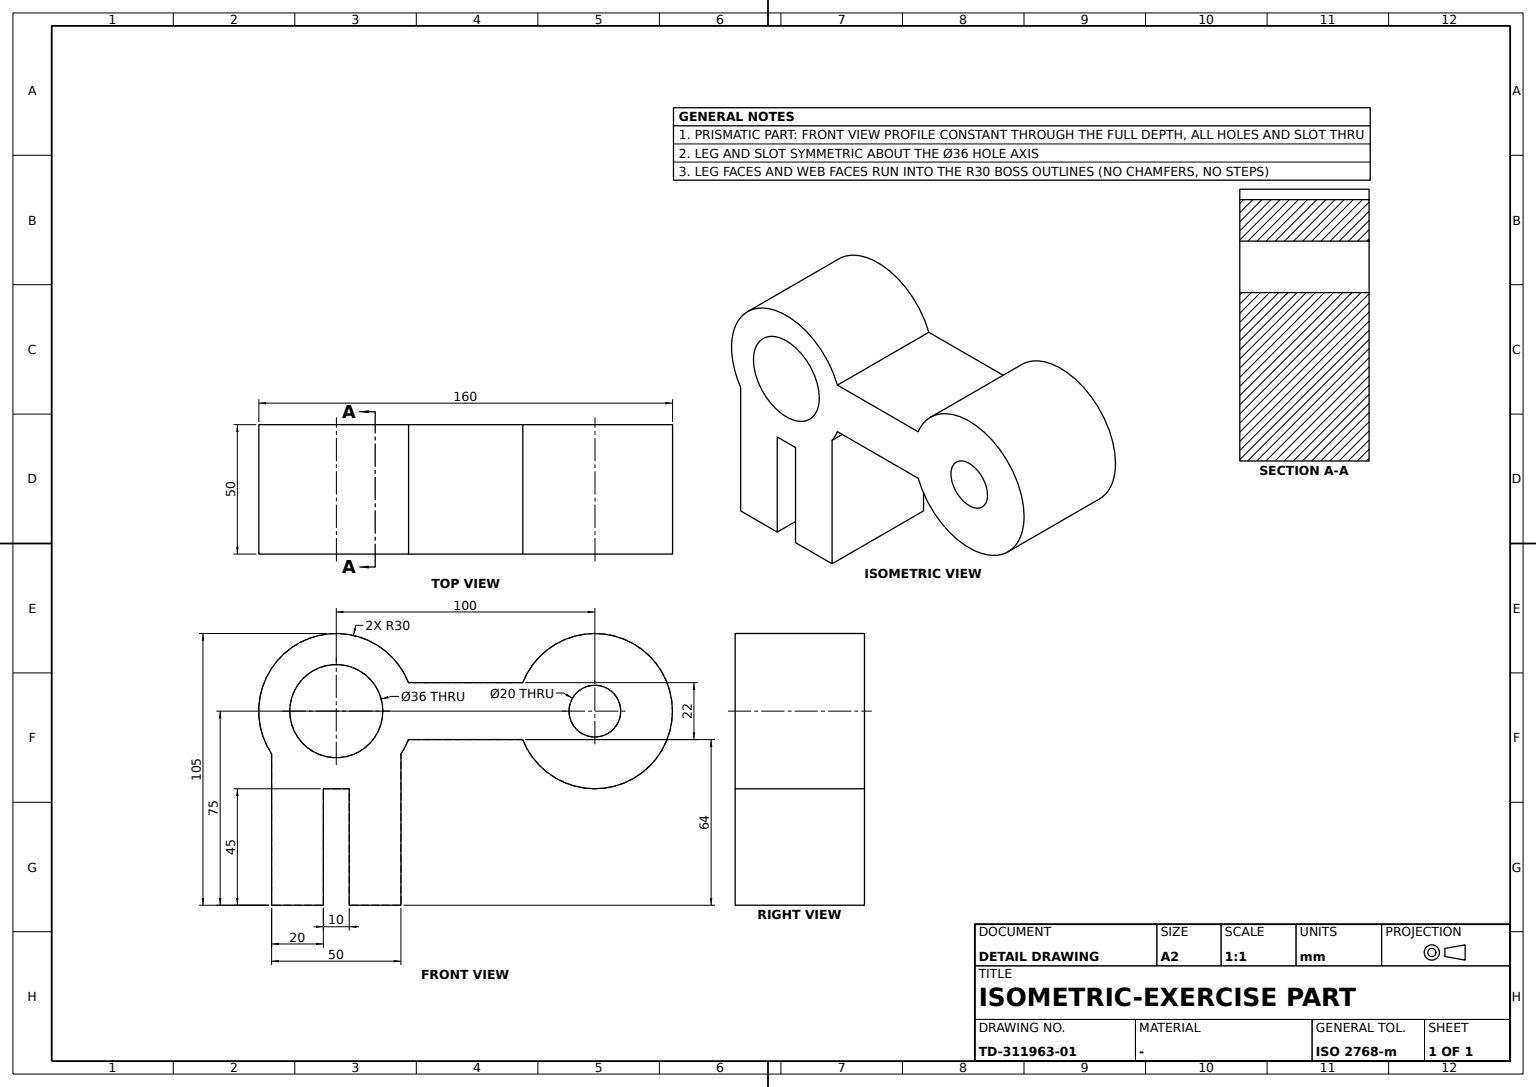
CATIA V5 part; units mm, degrees
sketch "Sketch1" plane through (0, 0, 0) normal (1, 0, 0) x (0, 1, 0)
  arc A0 (25, -16.5831) -> (-25, -16.5831) centre (0, 0) ccw
  circle A1 centre (0, 0) radius 18
  line L0 (-25, -75) -> (-5, -75)
  line L1 (25, -75) -> (25, -16.5831)
  line L2 (5, -30) -> (-5, -30)
  line L3 (-5, -30) -> (-5, -75)
  line L4 (5, -30) -> (5, -75)
  point P0 (5, -75)
  line L5 (5, -75) -> (25, -75)
  line L6 (-25, -75) -> (-25, -16.5831)
  dimension "radius A0" = 30
  dimension "radius A1" = 18
  dimension "distance L4 L1" = 20
  dimension "distance L6 L1" = 50
  dimension "distance L6 L3" = 20
  dimension "distance L2 L0" = 45
  dimension "distance origin L0" = 75
  constraint horizontal L0 x-axis
  constraint horizontal L2 x-axis
  constraint horizontal L5 x-axis
  constraint vertical L1 y-axis
  constraint vertical L3 y-axis
  constraint vertical L4 y-axis
  constraint coincidence P0 L0
  constraint coincidence L0 L5
  constraint symmetry L3 L4 y-axis
extrude "Pad1" add sketch "Sketch1" along normal mid plane 50
sketch "Sketch2" plane through (0, 0, 0) normal (1, 0, 0) x (0, 1, 0)
  circle A0 centre (100, 0) radius 10
  point P0 (100, 0)
  circle A1 centre (100, 0) radius 30
  arc A2 (25, -16.5831) -> (-25, -16.5831) centre (0, 0) ccw construction
  dimension "radius A0" = 10
  dimension "distance origin P0" = 100
  constraint coincidence P0 x-axis
  constraint equal size A2 A1
extrude "Pad2" add sketch "Sketch2" along normal mid plane 50
sketch "Sketch3" plane through (0, 0, 0) normal (1, 0, 0) x (0, 1, 0)
  circle A0 centre (100, 0) radius 30 construction
  arc A1 (72.0894, 11) -> (72.0894, -11) centre (100, 0) ccw
  arc A2 (25, -16.5831) -> (-25, -16.5831) centre (0, 0) ccw construction
  arc A3 (27.9106, -11) -> (27.9106, 11) centre (0, 0) ccw
  point P0 (27.9106, 11)
  line L0 (27.9106, 11) -> (72.0894, 11)
  point P1 (72.0894, 11)
  point P2 (27.9106, -11)
  line L1 (27.9106, -11) -> (72.0894, -11)
  point P3 (72.0894, -11)
  dimension "distance L0 L1" = 22
  constraint coincidence P0 A2
  constraint coincidence P1 A0
  constraint coincidence P2 A2
  constraint coincidence P3 A0
  constraint horizontal L0 x-axis
  constraint horizontal L1 x-axis
  constraint symmetry L0 L1 x-axis
extrude "Pad3" add sketch "Sketch3" along normal mid plane 50
properties part number "Dual Cylindrical Boss Component with Slotted Vertical Base"
